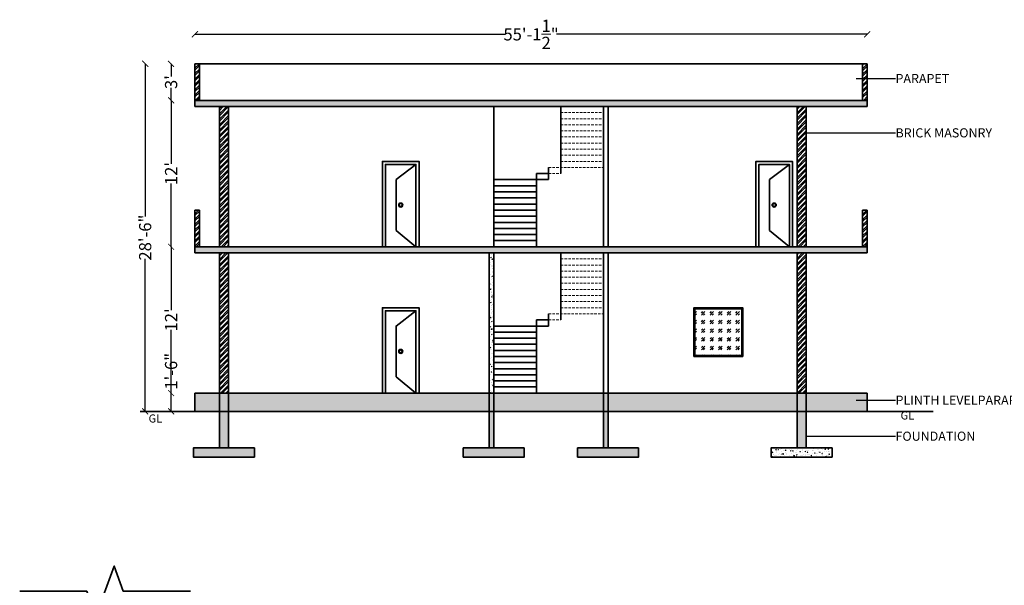
# Model space of a CAD drawing. Units: inches. Extents: x 626 to 5030, y -1681 to 1720.
# Tile 3 of 5: x 2191 to 3160, y 1163 to 1720. Entities that reach past the tile are written whole.
import ezdxf
from ezdxf import colors
from ezdxf.entities.mleader import LeaderData, LeaderLine
from ezdxf.math import Vec2, Vec3

# ---------------------------------------------------------------- set-up
doc = ezdxf.new("R2010")
doc.units = ezdxf.units.IN
doc.header["$MEASUREMENT"] = 0
doc.linetypes.add('HIDDENX2', pattern=[0.75, 0.5, -0.25])
for name, color, linetype, lineweight in [('A-ANNO-DIMS', 2, 'Continuous', 18), ('A-ANNO-TEXT', 7, 'Continuous', 18), ('A-GLAZ', 4, 'Continuous', 25), ('A-SECT', 7, 'Continuous', 35), ('A-SECT-HIDN', 8, 'HIDDENX2', 18), ('A-SECT-PATT', 251, 'Continuous', 13), ('C-PROP', 1, 'Continuous', 35)]:
    doc.layers.add(name, color=color, linetype=linetype, lineweight=lineweight)
doc.styles.get("Standard").update_dxf_attribs({"font": 'arial.ttf'})
doc.dimstyles.get("Standard").update_dxf_attribs({"dimtxt": 12, "dimasz": 6, "dimexe": 0.18, "dimexo": 0.0625, "dimgap": 0.09, "dimtad": 0, "dimdec": 1, "dimzin": 0, "dimdsep": 46, "dimlunit": 4, "dimtxsty": 'Standard', "dimblk": 'ARCHTICK', "dimcen": 0.09, "dimse1": 1, "dimse2": 1, "dimclrt": 3, "dimadec": 0, "dimazin": 0, "dimtfac": 1, "dimtdec": 1, "dimtofl": 0, "dimtmove": 0, "dimatfit": 3, "dimfxl": 1, "dimtolj": 1, "dimtzin": 0, "dimarcsym": 0})
pattern_1 = [(50, (-956.896, -242.5), (7.172602, -0.627521), [0.75, -8.25]), (355, (-956.896, -242.5), (-1.387513, 7.521921), [0.6, -6.6]), (100.45144, (-956.2984, -242.552), (5.785088, 6.8944), [0.637402, -7.011421]), (46.1842, (-956.896, -240.5), (10.672413, -1.655193), [1.125, -12.375]), (96.63564, (-956.007, -240.638), (9.34662, 9.741186), [0.956103, -10.517138]), (351.18416, (-956.896, -240.5), (9.34662, 9.741186), [0.9, -9.9]), (21, (-955.896, -241), (5.9690705, -4.026189), [0.75, -8.25]), (326, (-955.896, -241), (2.433153, 7.2515), [0.6, -6.6]), (71.45144, (-955.3987, -241.3355), (8.402224, 3.225312), [0.637402, -7.011421]), (37.5, (-956.896, -242.5), (0.1215986, 3.3289385), [0, -6.52, 0, -6.7, 0, -6.625]), (7.5, (-956.896, -242.5), (2.6306954, 3.944117), [0, -3.82, 0, -6.37, 0, -2.525]), (327.5, (-959.126, -242.5), (5.3382244, -0.2255487), [0, -2.5, 0, -7.8, 0, -10.35]), (317.5, (-960.126, -242.5), (5.8318617, 1.00105), [0, -3.25, 0, -5.18, 0, -7.35])]
pattern_2 = [(45, (-956.896, -242.5), (-2.6516504, 2.6516504), []), (45, (-955.1283, -242.5), (-2.6516504, 2.6516504), [])]

# ---------------------------------------------------------------- blocks, each defined once
blk = doc.blocks.new('_ArchTick')
at = {"color": 0, "linetype": 'ByBlock', "const_width": 0.15}
blk.add_lwpolyline([(-0.5, -0.5), (0.5, 0.5)], dxfattribs=at)
blk = doc.blocks.new('*D39')
at = {"layer": 'A-ANNO-DIMS', "color": 0, "lineweight": -2, "transparency": 16777216}
for p, q in [((2339.6, 1352.5), (2339.6, 1358.5)), ((2339.6, 1334.5), (2339.6, 1352.5))]:
    blk.add_line(p, q, dxfattribs=at)
at = {"layer": 'DEFPOINTS', "color": 0, "transparency": 16777216}
for p in [(2339.6, 1352.5), (2363.1, 1352.5), (2363.1, 1334.5)]:
    blk.add_point(p, dxfattribs=at)
at = {"layer": 'A-ANNO-DIMS', "color": 0, "lineweight": -2, "transparency": 16777216, "xscale": 6, "yscale": 6, "zscale": 6}
for p, rotation in [((2339.6, 1352.5), 90), ((2339.6, 1334.5), 270)]:
    blk.add_blockref('_ArchTick', p, dxfattribs=dict(at, rotation=rotation))
at = {"layer": 'A-ANNO-DIMS', "color": 0, "transparency": 16777216, "insert": (2339.6, 1373.97), "char_height": 12, "attachment_point": 5, "rotation": 90}
blk.add_mtext('\\A1;1\'-6"', dxfattribs=at)
blk = doc.blocks.new('*D40')
at = {"layer": 'A-ANNO-DIMS', "color": 0, "lineweight": -2, "transparency": 16777216}
for p, q in [((2339.6, 1496.5), (2339.6, 1434.21)), ((2339.6, 1352.5), (2339.6, 1414.79))]:
    blk.add_line(p, q, dxfattribs=at)
at = {"layer": 'DEFPOINTS', "color": 0, "transparency": 16777216}
for p in [(2339.6, 1496.5), (2363.1, 1496.5), (2363.1, 1352.5)]:
    blk.add_point(p, dxfattribs=at)
at = {"layer": 'A-ANNO-DIMS', "color": 0, "lineweight": -2, "transparency": 16777216, "xscale": 6, "yscale": 6, "zscale": 6}
for p, rotation in [((2339.6, 1496.5), 90), ((2339.6, 1352.5), 270)]:
    blk.add_blockref('_ArchTick', p, dxfattribs=dict(at, rotation=rotation))
at = {"layer": 'A-ANNO-DIMS', "color": 0, "transparency": 16777216, "insert": (2339.6, 1424.5), "char_height": 12, "attachment_point": 5, "rotation": 90}
blk.add_mtext("\\A1;12'", dxfattribs=at)
blk = doc.blocks.new('*D41')
at = {"layer": 'A-ANNO-DIMS', "color": 0, "lineweight": -2, "transparency": 16777216}
for p, q in [((2339.6, 1640.5), (2339.6, 1578.21)), ((2339.6, 1496.5), (2339.6, 1558.79))]:
    blk.add_line(p, q, dxfattribs=at)
at = {"layer": 'DEFPOINTS', "color": 0, "transparency": 16777216}
for p in [(2339.6, 1640.5), (2363.1, 1640.5), (2363.1, 1496.5)]:
    blk.add_point(p, dxfattribs=at)
at = {"layer": 'A-ANNO-DIMS', "color": 0, "lineweight": -2, "transparency": 16777216, "xscale": 6, "yscale": 6, "zscale": 6}
for p, rotation in [((2339.6, 1640.5), 90), ((2339.6, 1496.5), 270)]:
    blk.add_blockref('_ArchTick', p, dxfattribs=dict(at, rotation=rotation))
at = {"layer": 'A-ANNO-DIMS', "color": 0, "transparency": 16777216, "insert": (2339.6, 1568.5), "char_height": 12, "attachment_point": 5, "rotation": 90}
blk.add_mtext("\\A1;12'", dxfattribs=at)
blk = doc.blocks.new('*D42')
at = {"layer": 'A-ANNO-DIMS', "color": 0, "lineweight": -2, "transparency": 16777216}
for p, q in [((2339.6, 1676.5), (2339.6, 1664.11)), ((2339.6, 1640.5), (2339.6, 1652.89))]:
    blk.add_line(p, q, dxfattribs=at)
at = {"layer": 'DEFPOINTS', "color": 0, "transparency": 16777216}
for p in [(2339.6, 1676.5), (2363.1, 1676.5), (2363.1, 1640.5)]:
    blk.add_point(p, dxfattribs=at)
at = {"layer": 'A-ANNO-DIMS', "color": 0, "lineweight": -2, "transparency": 16777216, "xscale": 6, "yscale": 6, "zscale": 6}
for p, rotation in [((2339.6, 1676.5), 90), ((2339.6, 1640.5), 270)]:
    blk.add_blockref('_ArchTick', p, dxfattribs=dict(at, rotation=rotation))
at = {"layer": 'A-ANNO-DIMS', "color": 0, "transparency": 16777216, "insert": (2339.6, 1658.5), "char_height": 12, "attachment_point": 5, "rotation": 90}
blk.add_mtext("\\A1;3'", dxfattribs=at)
blk = doc.blocks.new('*D43')
at = {"layer": 'A-ANNO-DIMS', "color": 0, "lineweight": -2, "transparency": 16777216}
for p, q in [((2314.1, 1676.5), (2314.1, 1526.3)), ((2314.1, 1334.5), (2314.1, 1484.7))]:
    blk.add_line(p, q, dxfattribs=at)
at = {"layer": 'DEFPOINTS', "color": 0, "transparency": 16777216}
for p in [(2363.1, 1676.5), (2314.1, 1334.5), (2363.1, 1334.5)]:
    blk.add_point(p, dxfattribs=at)
at = {"layer": 'A-ANNO-DIMS', "color": 0, "lineweight": -2, "transparency": 16777216, "xscale": 6, "yscale": 6, "zscale": 6}
for p, rotation in [((2314.1, 1676.5), 90), ((2314.1, 1334.5), 270)]:
    blk.add_blockref('_ArchTick', p, dxfattribs=dict(at, rotation=rotation))
at = {"layer": 'A-ANNO-DIMS', "color": 0, "transparency": 16777216, "insert": (2314.1, 1505.5), "char_height": 12, "attachment_point": 5, "rotation": 90}
blk.add_mtext('\\A1;28\'-6"', dxfattribs=at)
blk = doc.blocks.new('*D49')
at = {"layer": 'A-ANNO-DIMS', "color": 0, "lineweight": -2, "transparency": 16777216}
for p, q in [((2363.1, 1705.5), (2668.78, 1705.5)), ((3024.6, 1705.5), (2718.93, 1705.5))]:
    blk.add_line(p, q, dxfattribs=at)
at = {"layer": 'DEFPOINTS', "color": 0, "transparency": 16777216}
for p in [(3024.6, 1705.5), (2363.1, 1676.5), (3024.6, 1676.5)]:
    blk.add_point(p, dxfattribs=at)
at = {"layer": 'A-ANNO-DIMS', "color": 0, "lineweight": -2, "transparency": 16777216, "xscale": 6, "yscale": 6, "zscale": 6, "rotation": 180}
blk.add_blockref('_ArchTick', (2363.1, 1705.5), dxfattribs=at)
at = {"layer": 'A-ANNO-DIMS', "color": 0, "lineweight": -2, "transparency": 16777216, "xscale": 6, "yscale": 6, "zscale": 6}
blk.add_blockref('_ArchTick', (3024.6, 1705.5), dxfattribs=at)
at = {"layer": 'A-ANNO-DIMS', "color": 0, "transparency": 16777216, "insert": (2693.85, 1705.5), "char_height": 12, "attachment_point": 5}
blk.add_mtext('\\A1;55\'-1{\\H1x;\\S1/2;}"', dxfattribs=at)

msp = doc.modelspace()

# ---------------------------------------------------------------- hatches: boundary and pattern name
at = {"layer": 'A-GLAZ'}
h = msp.add_hatch(dxfattribs=at)
h.set_pattern_fill('GOST_GLASS', color=256)
h.set_pattern_definition([(45, (-956.896, -242.5), (8.485281, 0), [5, -7]), (45, (-954.775, -242.5), (8.485281, 0), [2, -10]), (45, (-956.896, -240.3787), (8.485281, 0), [2, -10])])
h.paths.add_polyline_path([(2901.17, 1435.5), (2855.17, 1435.5), (2855.17, 1389.5), (2901.17, 1389.5)])
at = {"layer": 'A-SECT-PATT'}
h = msp.add_hatch(dxfattribs=at)
h.set_pattern_fill('ANSI32', color=256, scale=10)
h.set_pattern_definition(pattern_2)
h.paths.add_polyline_path([(2367.6, 1532.5), (2363.1, 1532.5), (2363.1, 1496.5), (2367.6, 1496.5)])
h.paths.add_polyline_path([(3024.6, 1532.5), (3020.1, 1532.5), (3020.1, 1496.5), (3024.6, 1496.5)])
h.paths.add_polyline_path([(3024.6, 1676.5), (3020.1, 1676.5), (3020.1, 1640.5), (3024.6, 1640.5)])
h.paths.add_polyline_path([(2367.6, 1676.5), (2363.1, 1676.5), (2363.1, 1640.5), (2367.6, 1640.5)])
h = msp.add_hatch(dxfattribs=at)
h.set_pattern_fill('AR-CONC', color=256)
h.set_pattern_definition(pattern_1)
h.paths.add_polyline_path([(3024.6, 1640.5), (2363.1, 1640.5), (2363.1, 1634.5), (3024.6, 1634.5)])
h = msp.add_hatch(dxfattribs=at)
h.set_pattern_fill('ANSI32', color=256, scale=10)
h.set_pattern_definition(pattern_2)
h.paths.add_polyline_path([(2396.1, 1634.5), (2387.1, 1634.5), (2387.1, 1496.5), (2396.1, 1496.5)])
h.paths.add_polyline_path([(2396.1, 1490.5), (2387.1, 1490.5), (2387.1, 1352.5), (2396.1, 1352.5)])
h.paths.add_polyline_path([(2964.6, 1634.5), (2955.6, 1634.5), (2955.6, 1496.5), (2964.6, 1496.5)])
h.paths.add_polyline_path([(2964.6, 1490.5), (2955.6, 1490.5), (2955.6, 1352.5), (2964.6, 1352.5)])
h = msp.add_hatch(dxfattribs=at)
h.set_pattern_fill('AR-CONC', color=256)
h.set_pattern_definition(pattern_1)
h.paths.add_polyline_path([(3024.6, 1496.5), (2363.1, 1496.5), (2363.1, 1490.5), (3024.6, 1490.5)])
h = msp.add_hatch(dxfattribs=at)
h.set_pattern_fill('AR-CONC', color=256)
h.set_pattern_definition(pattern_1)
h.paths.add_polyline_path([(2657.1, 1490.5), (2652.6, 1490.5), (2652.6, 1352.5), (2657.1, 1352.5)])
h = msp.add_hatch(dxfattribs=at)
h.set_pattern_fill('AR-CONC', color=256)
h.set_pattern_definition(pattern_1)
h.paths.add_polyline_path([(2652.6, 1352.5), (2396.1, 1352.5), (2396.1, 1334.5), (2652.6, 1334.5)])
h.paths.add_polyline_path([(2387.1, 1352.5), (2363.1, 1352.5), (2363.1, 1334.5), (2387.1, 1334.5)])
h.paths.add_polyline_path([(2396.1, 1352.5), (2387.1, 1352.5), (2387.1, 1334.5), (2396.1, 1334.5)])
h.paths.add_polyline_path([(2396.1, 1334.5), (2387.1, 1334.5), (2387.1, 1298.5), (2396.1, 1298.5)])
h.paths.add_polyline_path([(2421.6, 1298.5), (2361.6, 1298.5), (2361.6, 1289.5), (2421.6, 1289.5)])
h.paths.add_polyline_path([(2765.1, 1352.5), (2657.1, 1352.5), (2657.1, 1334.5), (2765.1, 1334.5)])
h.paths.add_polyline_path([(2955.6, 1352.5), (2769.6, 1352.5), (2769.6, 1334.5), (2955.6, 1334.5)])
h.paths.add_polyline_path([(2964.6, 1352.5), (2955.6, 1352.5), (2955.6, 1334.5), (2964.6, 1334.5)])
h.paths.add_polyline_path([(3024.6, 1352.5), (2964.6, 1352.5), (2964.6, 1334.5), (3024.6, 1334.5)])
h.paths.add_polyline_path([(2964.6, 1334.5), (2955.6, 1334.5), (2955.6, 1298.5), (2964.6, 1298.5)])
h.paths.add_polyline_path([(2769.6, 1334.5), (2765.1, 1334.5), (2765.1, 1298.5), (2769.6, 1298.5)])
h.paths.add_polyline_path([(2657.1, 1334.5), (2652.6, 1334.5), (2652.6, 1298.5), (2657.1, 1298.5)])
h.paths.add_polyline_path([(2687.1, 1298.5), (2627.1, 1298.5), (2627.1, 1289.5), (2687.1, 1289.5)])
h.paths.add_polyline_path([(2799.6, 1298.5), (2739.6, 1298.5), (2739.6, 1289.5), (2799.6, 1289.5)])
h.paths.add_polyline_path([(2769.6, 1352.5), (2765.1, 1352.5), (2765.1, 1334.5), (2769.6, 1334.5)])
h.paths.add_polyline_path([(2657.1, 1352.5), (2652.6, 1352.5), (2652.6, 1334.5), (2657.1, 1334.5)])
h = msp.add_hatch(dxfattribs=at)
h.set_pattern_fill('AR-CONC', color=256)
h.set_pattern_definition(pattern_1)
h.paths.add_polyline_path([(2990.1, 1289.5), (2990.1, 1298.5), (2930.1, 1298.5), (2930.1, 1289.5)])

# ---------------------------------------------------------------- linework, layer by layer
at = {"layer": 'A-SECT'}
for p, q in [((2363.1, 1676.5), (3024.6, 1676.5)), ((2363.1, 1634.5), (2363.1, 1676.5)), ((2367.6, 1640.5), (2367.6, 1676.5)), ((3020.1, 1640.5), (3020.1, 1676.5)), ((3024.6, 1634.5), (3024.6, 1676.5)), ((2363.1, 1640.5), (3024.6, 1640.5)), ((2363.1, 1634.5), (3024.6, 1634.5)), ((2387.1, 1496.5), (2387.1, 1634.5)), ((2396.1, 1496.5), (2396.1, 1634.5)), ((2657.1, 1496.5), (2657.1, 1634.5)), ((2723.1, 1634.5), (2723.1, 1568.5)), ((2765.1, 1496.5), (2765.1, 1634.5)), ((2769.6, 1496.5), (2769.6, 1634.5)), ((2955.6, 1496.5), (2955.6, 1634.5)), ((2964.6, 1496.5), (2964.6, 1634.5)), ((2711.1, 1562.5), (2711.1, 1574.5)), ((2699.1, 1562.5), (2657.1, 1562.5)), ((2699.1, 1568.5), (2711.1, 1568.5)), ((2699.1, 1568.5), (2699.1, 1496.5)), ((2699.1, 1562.5), (2711.1, 1562.5)), ((2699.1, 1556.5), (2657.1, 1556.5)), ((2699.1, 1550.5), (2657.1, 1550.5)), ((2699.1, 1544.5), (2657.1, 1544.5)), ((2363.1, 1490.5), (2363.1, 1532.5)), ((2363.1, 1532.5), (2367.6, 1532.5)), ((2367.6, 1496.5), (2367.6, 1532.5)), ((2699.1, 1538.5), (2657.1, 1538.5)), ((2699.1, 1532.5), (2657.1, 1532.5)), ((3020.1, 1496.5), (3020.1, 1532.5)), ((3020.1, 1532.5), (3024.6, 1532.5)), ((3024.6, 1490.5), (3024.6, 1532.5)), ((2699.1, 1526.5), (2657.1, 1526.5)), ((2699.1, 1520.5), (2657.1, 1520.5)), ((2699.1, 1514.5), (2657.1, 1514.5)), ((2699.1, 1508.5), (2657.1, 1508.5)), ((2699.1, 1502.5), (2657.1, 1502.5)), ((2363.1, 1496.5), (3024.6, 1496.5)), ((2363.1, 1490.5), (2363.1, 1496.5)), ((3024.6, 1490.5), (3024.6, 1496.5)), ((2363.1, 1490.5), (3024.6, 1490.5)), ((2387.1, 1298.5), (2387.1, 1490.5)), ((2396.1, 1298.5), (2396.1, 1490.5)), ((2652.6, 1298.5), (2652.6, 1490.5)), ((2657.1, 1298.5), (2657.1, 1490.5)), ((2723.1, 1490.5), (2723.1, 1424.5)), ((2765.1, 1298.5), (2765.1, 1490.5)), ((2769.6, 1298.5), (2769.6, 1490.5)), ((2955.6, 1298.5), (2955.6, 1490.5)), ((2964.6, 1298.5), (2964.6, 1490.5)), ((2699.1, 1424.5), (2711.1, 1424.5)), ((2699.1, 1424.5), (2699.1, 1352.5)), ((2711.1, 1418.5), (2711.1, 1430.5)), ((2699.1, 1418.5), (2657.1, 1418.5)), ((2699.1, 1418.5), (2711.1, 1418.5)), ((2699.1, 1412.5), (2657.1, 1412.5)), ((2699.1, 1406.5), (2657.1, 1406.5)), ((2699.1, 1400.5), (2657.1, 1400.5)), ((2699.1, 1394.5), (2657.1, 1394.5)), ((2699.1, 1388.5), (2657.1, 1388.5)), ((2699.1, 1382.5), (2657.1, 1382.5)), ((2699.1, 1376.5), (2657.1, 1376.5)), ((2699.1, 1370.5), (2657.1, 1370.5)), ((2699.1, 1364.5), (2657.1, 1364.5)), ((2699.1, 1358.5), (2657.1, 1358.5)), ((2363.1, 1352.5), (3024.6, 1352.5)), ((2363.1, 1334.5), (2363.1, 1352.5)), ((3024.6, 1334.5), (3024.6, 1352.5)), ((2309.1, 1334.5), (3089.6, 1334.5)), ((2387.1, 1298.5), (2396.1, 1298.5))]:
    msp.add_line(p, q, dxfattribs=at)
for points in [[(2547.6, 1496.5), (2547.6, 1580.5), (2583.6, 1580.5), (2583.6, 1496.5)], [(2951.1, 1496.5), (2951.1, 1580.5), (2915.1, 1580.5), (2915.1, 1496.5)], [(2550.6, 1496.5), (2550.6, 1577.5), (2580.6, 1577.5), (2580.6, 1496.5), (2561.1, 1512.5), (2561.1, 1562.5), (2580.6, 1577.5)], [(2948.1, 1496.5), (2948.1, 1577.5), (2918.1, 1577.5), (2918.1, 1496.5)], [(2918.1, 1496.5), (2918.1, 1577.5), (2948.1, 1577.5), (2948.1, 1496.5), (2928.6, 1512.5), (2928.6, 1562.5), (2948.1, 1577.5)], [(2547.6, 1352.5), (2547.6, 1436.5), (2583.6, 1436.5), (2583.6, 1352.5)], [(2550.6, 1352.5), (2550.6, 1433.5), (2580.6, 1433.5), (2580.6, 1352.5), (2561.1, 1368.5), (2561.1, 1418.5), (2580.6, 1433.5)]]:
    msp.add_lwpolyline(points, dxfattribs=at)
for points in [[(2902.17, 1388.5), (2854.17, 1388.5), (2854.17, 1436.5), (2902.17, 1436.5)], [(2901.17, 1389.5), (2855.17, 1389.5), (2855.17, 1435.5), (2901.17, 1435.5)], [(2421.6, 1298.5), (2421.6, 1289.5), (2361.6, 1289.5), (2361.6, 1298.5)], [(2687.1, 1298.5), (2687.1, 1289.5), (2627.1, 1289.5), (2627.1, 1298.5)], [(2799.6, 1298.5), (2799.6, 1289.5), (2739.6, 1289.5), (2739.6, 1298.5)], [(2990.1, 1298.5), (2990.1, 1289.5), (2930.1, 1289.5), (2930.1, 1298.5)]]:
    msp.add_lwpolyline(points, close=True, dxfattribs=at)
for centre, radius in [((2565.6, 1537.5), 2), ((2565.6, 1537.5), 1.5), ((2933.1, 1537.5), 2), ((2933.1, 1537.5), 1.5), ((2565.6, 1393.5), 2), ((2565.6, 1393.5), 1.5)]:
    msp.add_circle(centre, radius, dxfattribs=at)
at = {"layer": 'A-SECT-HIDN', "ltscale": 5}
for p, q in [((2723.1, 1628.5), (2765.1, 1628.5)), ((2723.1, 1622.5), (2765.1, 1622.5)), ((2723.1, 1616.5), (2765.1, 1616.5)), ((2723.1, 1610.5), (2765.1, 1610.5)), ((2723.1, 1604.5), (2765.1, 1604.5)), ((2723.1, 1598.5), (2765.1, 1598.5)), ((2723.1, 1592.5), (2765.1, 1592.5)), ((2723.1, 1586.5), (2765.1, 1586.5)), ((2723.1, 1580.5), (2765.1, 1580.5)), ((2711.1, 1574.5), (2765.1, 1574.5)), ((2711.1, 1568.5), (2723.1, 1568.5)), ((2723.1, 1484.5), (2765.1, 1484.5)), ((2723.1, 1478.5), (2765.1, 1478.5)), ((2723.1, 1472.5), (2765.1, 1472.5)), ((2723.1, 1466.5), (2765.1, 1466.5)), ((2723.1, 1460.5), (2765.1, 1460.5)), ((2723.1, 1454.5), (2765.1, 1454.5)), ((2723.1, 1448.5), (2765.1, 1448.5)), ((2723.1, 1442.5), (2765.1, 1442.5)), ((2723.1, 1436.5), (2765.1, 1436.5)), ((2711.1, 1430.5), (2765.1, 1430.5)), ((2711.1, 1424.5), (2723.1, 1424.5))]:
    msp.add_line(p, q, dxfattribs=at)
at = {"layer": 'C-PROP'}
msp.add_lwpolyline([(2190.6, 1157.57), (2256.6, 1157.57), (2265.6, 1132.84), (2283.6, 1182.29), (2292.6, 1157.57), (2358.6, 1157.57)], dxfattribs=at)

# ---------------------------------------------------------------- texts
at = {"layer": 'A-ANNO-TEXT', "char_height": 8, "attachment_point": 1}
for insert in [(2308.27, 1331.5), (3048.27, 1334.5)]:
    msp.add_mtext_dynamic_manual_height_columns('\\pxqc;GL', width=31.8381, gutter_width=1, heights=[0], dxfattribs=dict(at, insert=insert))

# ---------------------------------------------------------------- dimensions: what is measured, and where the dimension line sits
at = {"layer": 'A-ANNO-DIMS'}
dim = msp.add_linear_dim(base=(3024.6, 1705.5), p1=(2363.1, 1676.5), p2=(3024.6, 1676.5), dimstyle='Standard', override={"dimclrd": 0, "dimclre": 0, "dimclrt": 0}, dxfattribs=at)
dim.commit()
dim.dimension.update_dxf_attribs({"geometry": '*D49', "text_midpoint": (2693.85, 1705.5)})
for base, p1, p2, picture, middle in [((2314.1, 1334.5), (2363.1, 1676.5), (2363.1, 1334.5), '*D43', (2314.1, 1505.5)), ((2339.6, 1676.5), (2363.1, 1640.5), (2363.1, 1676.5), '*D42', (2339.6, 1658.5)), ((2339.6, 1640.5), (2363.1, 1496.5), (2363.1, 1640.5), '*D41', (2339.6, 1568.5)), ((2339.6, 1496.5), (2363.1, 1352.5), (2363.1, 1496.5), '*D40', (2339.6, 1424.5)), ((2339.6, 1352.5), (2363.1, 1334.5), (2363.1, 1352.5), '*D39', (2339.6, 1373.97))]:
    dim = msp.add_linear_dim(base=base, p1=p1, p2=p2, angle=90, dimstyle='Standard', override={"dimclrd": 0, "dimclre": 0, "dimclrt": 0}, dxfattribs=at)
    dim.commit()
    dim.dimension.update_dxf_attribs({"geometry": picture, "text_midpoint": middle})

# ---------------------------------------------------------------- leaders
at = {"layer": 'A-ANNO-TEXT'}
ml = msp.add_multileader_mtext('Standard', dxfattribs=at)
ml.set_content('PARAPET', color=256)
ml.set_leader_properties()
ml.build(insert=Vec2(0, 0))
ml.multileader.update_dxf_attribs({"dogleg_length": 0.36, "arrow_head_size": 0.18})
ctx = ml.context
ctx.base_point, ctx.char_height, ctx.arrow_head_size, ctx.landing_gap_size, ctx.plane_origin = Vec3(3052.46, 1662), 9, 0.18, 0.09, Vec3(3013.6, 1662)
notes = []
notes.append((ctx, [(0, (1, 1, 0), (3052.1, 1662), (1, 0), 0.36, [(0, [(3013.6, 1662)], 0, [])])]))
ctx.mtext.insert, ctx.mtext.flow_direction = Vec3(3052.55, 1666.5), 5
ml = msp.add_multileader_mtext('Standard', dxfattribs=at)
ml.set_content('BRICK MASONRY', color=256)
ml.set_leader_properties()
ml.build(insert=Vec2(0, 0))
ml.multileader.update_dxf_attribs({"dogleg_length": 0.36, "arrow_head_size": 0.18})
ctx = ml.context
ctx.base_point, ctx.char_height, ctx.arrow_head_size, ctx.landing_gap_size, ctx.plane_origin = Vec3(3052.46, 1608.5), 9, 0.18, 0.09, Vec3(3013.6, 1608.5)
notes.append((ctx, [(0, (1, 1, 0), (3052.1, 1608.5), (1, 0), 0.36, [(0, [(2964.6, 1608.5)], 0, [])])]))
ctx.mtext.insert, ctx.mtext.flow_direction = Vec3(3052.55, 1613.08), 5
ml = msp.add_multileader_mtext('Standard', dxfattribs=at)
ml.set_content('PLINTH LEVELPARAPET', color=256)
ml.set_leader_properties()
ml.build(insert=Vec2(0, 0))
ml.multileader.update_dxf_attribs({"dogleg_length": 0.36, "arrow_head_size": 0.18})
ctx = ml.context
ctx.base_point, ctx.char_height, ctx.arrow_head_size, ctx.landing_gap_size, ctx.plane_origin = Vec3(3052.46, 1345.5), 9, 0.18, 0.09, Vec3(3013.6, 1345.5)
notes.append((ctx, [(0, (1, 1, 0), (3052.1, 1345.5), (1, 0), 0.36, [(0, [(3013.6, 1345.5)], 0, [])])]))
ctx.mtext.insert, ctx.mtext.flow_direction = Vec3(3052.55, 1350), 5
ml = msp.add_multileader_mtext('Standard', dxfattribs=at)
ml.set_content('FOUNDATION', color=256)
ml.set_leader_properties()
ml.build(insert=Vec2(0, 0))
ml.multileader.update_dxf_attribs({"dogleg_length": 0.36, "arrow_head_size": 0.18})
ctx = ml.context
ctx.base_point, ctx.char_height, ctx.arrow_head_size, ctx.landing_gap_size, ctx.plane_origin = Vec3(3052.46, 1310), 9, 0.18, 0.09, Vec3(3013.6, 1310)
notes.append((ctx, [(0, (1, 1, 0), (3052.1, 1310), (1, 0), 0.36, [(0, [(2964.6, 1310)], 0, [])])]))
ctx.mtext.insert, ctx.mtext.flow_direction = Vec3(3052.55, 1314.58), 5
for ctx, leaders in notes:
    for number, flags, end, landing, length, lines in leaders:
        leader = LeaderData()
        leader.index, (leader.has_last_leader_line, leader.has_dogleg_vector, leader.attachment_direction) = number, flags
        leader.last_leader_point, leader.dogleg_vector, leader.dogleg_length = Vec3(end), Vec3(landing), length
        for number, points, colour, breaks in lines:
            line = LeaderLine()
            line.index, line.vertices, line.color, line.breaks = number, Vec3.list(points), colors.encode_raw_color(colour), breaks
            leader.lines.append(line)
        ctx.leaders.append(leader)

doc.saveas('drawing.dxf')
